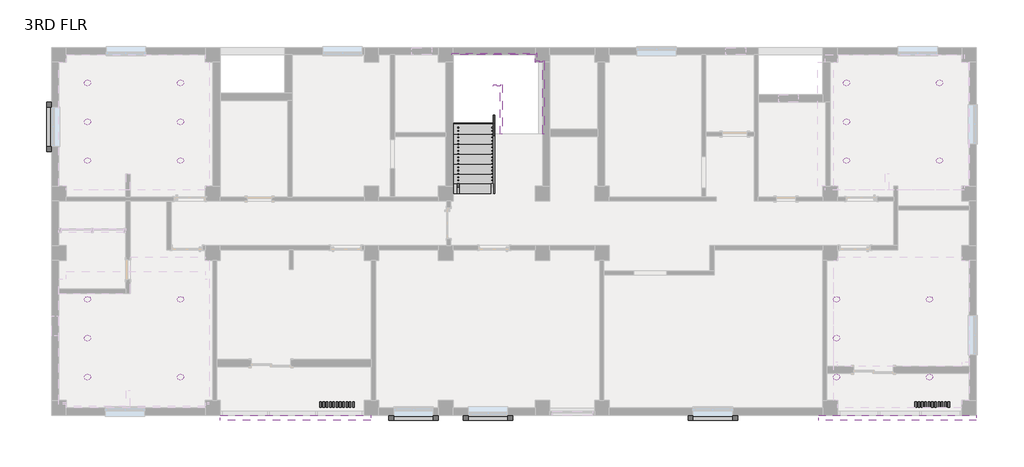
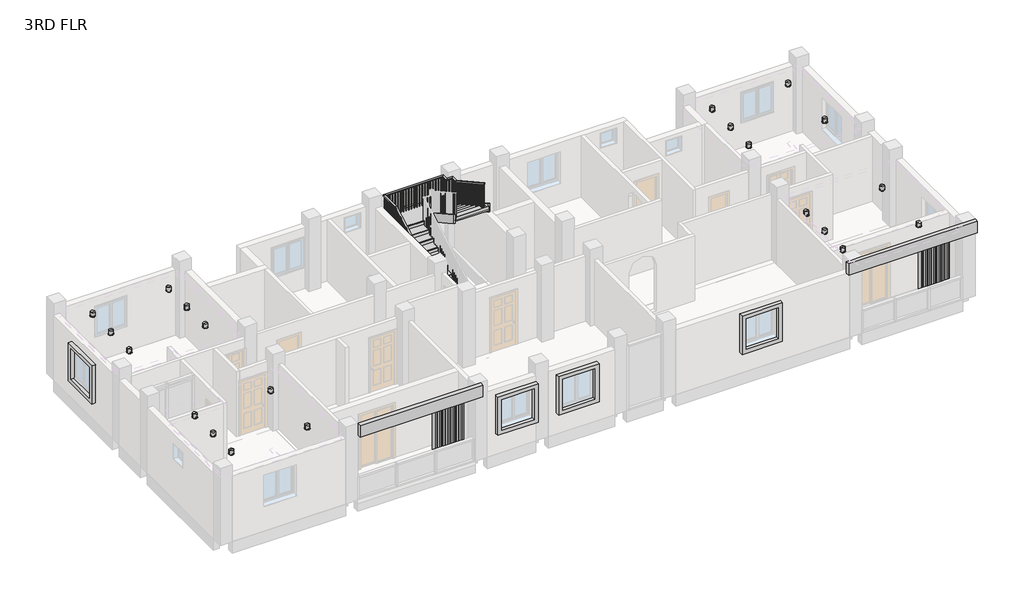
# One storey, part 5 of 5: 21 light fixtures, 8 members, 8 proxies, 1 railing, 1 stair flight.
"""IFC4 building model written with IfcOpenShell, lengths in millimetres."""

from ifc_helpers import new_model, si_unit, frame, origin, place, context, project, spatial, polyline, outline, extrude, faceted_brep, transform, mapped, element, save
from components import generic_models_11_generic_models_4_fdae65e2, generic_models_12_generic_models_6_f1297f64, generic_models_17_generic_models_17_4194431e, generic_models_21_generic_models_21_07dc1754, generic_models_4_generic_models_4_029e57d7, light_modern_pendant_14774_baffle_cc9af11b, light_modern_pendant_14774_baffle_b3430626, stair_flight_75ba705f

model = new_model("IFC4")

# Units and contexts
model_context = context("Model", 3, world=origin())
ifc_project = project(units=[si_unit("LENGTHUNIT", "METRE", prefix="MILLI")], contexts=[model_context])

# Site, building, storey
site = spatial("IfcSite", under=ifc_project)
building = spatial("IfcBuilding", under=site)
storey = spatial("IfcBuildingStorey", under=building, Name="3RD FLR", Elevation=9448.8)

# Proxies
placement = place(None, origin())
generic_models_11_generic_models_4_shape = generic_models_11_generic_models_4_fdae65e2(model_context)
element("IfcBuildingElementProxy", 1, Name="Generic Models 11 : Generic Models 4", ObjectType="Generic Models 11 : Generic Models 4", at=placement, inside=storey, context=model_context, shape_type="MappedRepresentation", body=[
    mapped(generic_models_11_generic_models_4_shape, transform((18611.1584144, 0.0, 0.0), x_axis=(1.0, 0.0, 0.0), y_axis=(0.0, 1.0, 0.0), z_axis=(0.0, 0.0, 1.0))),
])
generic_models_12_generic_models_6_shape = generic_models_12_generic_models_6_f1297f64(model_context)
element("IfcBuildingElementProxy", 2, Name="Generic Models 12 : Generic Models 6", ObjectType="Generic Models 12 : Generic Models 6", at=placement, inside=storey, context=model_context, shape_type="MappedRepresentation", body=[
    mapped(generic_models_12_generic_models_6_shape, transform((18288.0, 228.6, 0.0), x_axis=(1.0, 0.0, 0.0), y_axis=(0.0, 1.0, 0.0), z_axis=(0.0, 0.0, 1.0))),
])
generic_models_17_generic_models_17_shape = generic_models_17_generic_models_17_4194431e(model_context)
element("IfcBuildingElementProxy", 3, Name="Generic Models 17 : Generic Models 17", ObjectType="Generic Models 17 : Generic Models 17", at=placement, inside=storey, context=model_context, shape_type="MappedRepresentation", body=[
    mapped(generic_models_17_generic_models_17_shape, transform((0.0, 0.0, 0.0), x_axis=(1.0, 0.0, 0.0), y_axis=(0.0, 1.0, 0.0), z_axis=(0.0, 0.0, 1.0))),
])
generic_models_21_generic_models_21_shape = generic_models_21_generic_models_21_07dc1754(model_context)
element("IfcBuildingElementProxy", 4, Name="Generic Models 21 : Generic Models 21", ObjectType="Generic Models 21 : Generic Models 21", at=placement, inside=storey, context=model_context, shape_type="MappedRepresentation", body=[
    mapped(generic_models_21_generic_models_21_shape, transform((0.0, 0.0, 0.0), x_axis=(1.0, 0.0, 0.0), y_axis=(0.0, 1.0, 0.0), z_axis=(0.0, 0.0, 1.0))),
])
element("IfcBuildingElementProxy", 5, Name="Generic Models 25 : Generic Models 21", ObjectType="Generic Models 25 : Generic Models 21", at=placement, inside=storey, context=model_context, shape_type="MappedRepresentation", body=[
    mapped(generic_models_21_generic_models_21_shape, transform((-6905.3372689, 0.0, 0.0), x_axis=(1.0, 0.0, 0.0), y_axis=(0.0, 1.0, 0.0), z_axis=(0.0, 0.0, 1.0))),
])
element("IfcBuildingElementProxy", 6, Name="Generic Models 31 : Generic Models 21", ObjectType="Generic Models 31 : Generic Models 21", at=placement, inside=storey, context=model_context, shape_type="MappedRepresentation", body=[
    mapped(generic_models_21_generic_models_21_shape, transform((-9191.3372689, 0.0, 0.0), x_axis=(1.0, 0.0, 0.0), y_axis=(0.0, 1.0, 0.0), z_axis=(0.0, 0.0, 1.0))),
])
generic_models_4_generic_models_4_shape = generic_models_4_generic_models_4_029e57d7(model_context)
element("IfcBuildingElementProxy", 7, Name="Generic Models 4 : Generic Models 4", ObjectType="Generic Models 4 : Generic Models 4", at=placement, inside=storey, context=model_context, shape_type="MappedRepresentation", body=[
    mapped(generic_models_4_generic_models_4_shape, transform((0.0, 0.0, 0.0), x_axis=(1.0, 0.0, 0.0), y_axis=(0.0, 1.0, 0.0), z_axis=(0.0, 0.0, 1.0))),
])
element("IfcBuildingElementProxy", 8, Name="Generic Models 6 : Generic Models 6", ObjectType="Generic Models 6 : Generic Models 6", at=placement, inside=storey, context=model_context, shape_type="MappedRepresentation", body=[
    mapped(generic_models_12_generic_models_6_shape, transform((0.0, 228.6, 0.0), x_axis=(1.0, 0.0, 0.0), y_axis=(0.0, 1.0, 0.0), z_axis=(0.0, 0.0, 1.0))),
])

# Light fixtures
light_modern_pendant_14774_baffle_shape = light_modern_pendant_14774_baffle_cc9af11b(model_context)
element("IfcLightFixture", 9, ObjectType="LIGHT_-_MODERN_PENDANT_14774 : Baffle", at=placement, inside=storey, context=model_context, shape_type="MappedRepresentation", body=[
    mapped(light_modern_pendant_14774_baffle_shape, transform((-14269.0456086, -897.3794704, 9575.8), x_axis=(1.0, 0.0, 0.0), y_axis=(0.0, 1.0, 0.0), z_axis=(0.0, 0.0, 1.0))),
])
element("IfcLightFixture", 10, ObjectType="LIGHT_-_MODERN_PENDANT_14774 : Baffle", at=placement, inside=storey, context=model_context, shape_type="MappedRepresentation", body=[
    mapped(light_modern_pendant_14774_baffle_shape, transform((-14269.0456086, -3284.9794704, 9575.8), x_axis=(1.0, 0.0, 0.0), y_axis=(0.0, 1.0, 0.0), z_axis=(0.0, 0.0, 1.0))),
])
element("IfcLightFixture", 11, ObjectType="LIGHT_-_MODERN_PENDANT_14774 : Baffle", at=placement, inside=storey, context=model_context, shape_type="MappedRepresentation", body=[
    mapped(light_modern_pendant_14774_baffle_shape, transform((-14269.0456086, -2091.1794704, 9575.8), x_axis=(1.0, 0.0, 0.0), y_axis=(0.0, 1.0, 0.0), z_axis=(0.0, 0.0, 1.0))),
])
element("IfcLightFixture", 12, ObjectType="LIGHT_-_MODERN_PENDANT_14774 : Baffle", at=placement, inside=storey, context=model_context, shape_type="MappedRepresentation", body=[
    mapped(light_modern_pendant_14774_baffle_shape, transform((9048.1543914, -897.3794704, 9575.8), x_axis=(1.0, 0.0, 0.0), y_axis=(0.0, 1.0, 0.0), z_axis=(0.0, 0.0, 1.0))),
])
element("IfcLightFixture", 13, ObjectType="LIGHT_-_MODERN_PENDANT_14774 : Baffle", at=placement, inside=storey, context=model_context, shape_type="MappedRepresentation", body=[
    mapped(light_modern_pendant_14774_baffle_shape, transform((9048.1543914, -3284.9794704, 9575.8), x_axis=(1.0, 0.0, 0.0), y_axis=(0.0, 1.0, 0.0), z_axis=(0.0, 0.0, 1.0))),
])
element("IfcLightFixture", 14, ObjectType="LIGHT_-_MODERN_PENDANT_14774 : Baffle", at=placement, inside=storey, context=model_context, shape_type="MappedRepresentation", body=[
    mapped(light_modern_pendant_14774_baffle_shape, transform((9048.1543914, -2091.1794704, 9575.8), x_axis=(1.0, 0.0, 0.0), y_axis=(0.0, 1.0, 0.0), z_axis=(0.0, 0.0, 1.0))),
])
element("IfcLightFixture", 15, ObjectType="LIGHT_-_MODERN_PENDANT_14774 : Baffle", at=placement, inside=storey, context=model_context, shape_type="MappedRepresentation", body=[
    mapped(light_modern_pendant_14774_baffle_shape, transform((-14269.0456086, -7552.1794704, 9575.8), x_axis=(1.0, 0.0, 0.0), y_axis=(0.0, 1.0, 0.0), z_axis=(0.0, 0.0, 1.0))),
])
element("IfcLightFixture", 16, ObjectType="LIGHT_-_MODERN_PENDANT_14774 : Baffle", at=placement, inside=storey, context=model_context, shape_type="MappedRepresentation", body=[
    mapped(light_modern_pendant_14774_baffle_shape, transform((-14269.0456086, -9939.7794704, 9575.8), x_axis=(1.0, 0.0, 0.0), y_axis=(0.0, 1.0, 0.0), z_axis=(0.0, 0.0, 1.0))),
])
element("IfcLightFixture", 17, ObjectType="LIGHT_-_MODERN_PENDANT_14774 : Baffle", at=placement, inside=storey, context=model_context, shape_type="MappedRepresentation", body=[
    mapped(light_modern_pendant_14774_baffle_shape, transform((-14269.0456086, -8745.9794704, 9575.8), x_axis=(1.0, 0.0, 0.0), y_axis=(0.0, 1.0, 0.0), z_axis=(0.0, 0.0, 1.0))),
])
element("IfcLightFixture", 18, ObjectType="LIGHT_-_MODERN_PENDANT_14774 : Baffle", at=placement, inside=storey, context=model_context, shape_type="MappedRepresentation", body=[
    mapped(light_modern_pendant_14774_baffle_shape, transform((8743.3543914, -7552.1794704, 9575.8), x_axis=(1.0, 0.0, 0.0), y_axis=(0.0, 1.0, 0.0), z_axis=(0.0, 0.0, 1.0))),
])
element("IfcLightFixture", 19, ObjectType="LIGHT_-_MODERN_PENDANT_14774 : Baffle", at=placement, inside=storey, context=model_context, shape_type="MappedRepresentation", body=[
    mapped(light_modern_pendant_14774_baffle_shape, transform((8743.3543914, -9939.7794704, 9575.8), x_axis=(1.0, 0.0, 0.0), y_axis=(0.0, 1.0, 0.0), z_axis=(0.0, 0.0, 1.0))),
])
element("IfcLightFixture", 20, ObjectType="LIGHT_-_MODERN_PENDANT_14774 : Baffle", at=placement, inside=storey, context=model_context, shape_type="MappedRepresentation", body=[
    mapped(light_modern_pendant_14774_baffle_shape, transform((8743.3543914, -8745.9794704, 9575.8), x_axis=(1.0, 0.0, 0.0), y_axis=(0.0, 1.0, 0.0), z_axis=(0.0, 0.0, 1.0))),
])
light_modern_pendant_14774_baffle_2_shape = light_modern_pendant_14774_baffle_b3430626(model_context)
element("IfcLightFixture", 21, ObjectType="LIGHT_-_MODERN_PENDANT_14774 : Baffle", at=placement, inside=storey, context=model_context, shape_type="MappedRepresentation", body=[
    mapped(light_modern_pendant_14774_baffle_2_shape, transform((-11411.5456086, -897.3794704, 9575.8), x_axis=(-1.0, 0.0, 0.0), y_axis=(0.0, -1.0, 0.0), z_axis=(0.0, 0.0, 1.0))),
])
element("IfcLightFixture", 22, ObjectType="LIGHT_-_MODERN_PENDANT_14774 : Baffle", at=placement, inside=storey, context=model_context, shape_type="MappedRepresentation", body=[
    mapped(light_modern_pendant_14774_baffle_2_shape, transform((-11411.5456086, -3284.9794704, 9575.8), x_axis=(-1.0, 0.0, 0.0), y_axis=(0.0, -1.0, 0.0), z_axis=(0.0, 0.0, 1.0))),
])
element("IfcLightFixture", 23, ObjectType="LIGHT_-_MODERN_PENDANT_14774 : Baffle", at=placement, inside=storey, context=model_context, shape_type="MappedRepresentation", body=[
    mapped(light_modern_pendant_14774_baffle_2_shape, transform((-11411.5456086, -2091.1794704, 9575.8), x_axis=(-1.0, 0.0, 0.0), y_axis=(0.0, -1.0, 0.0), z_axis=(0.0, 0.0, 1.0))),
])
element("IfcLightFixture", 24, ObjectType="LIGHT_-_MODERN_PENDANT_14774 : Baffle", at=placement, inside=storey, context=model_context, shape_type="MappedRepresentation", body=[
    mapped(light_modern_pendant_14774_baffle_2_shape, transform((11905.6543914, -897.3794704, 9575.8), x_axis=(-1.0, 0.0, 0.0), y_axis=(0.0, -1.0, 0.0), z_axis=(0.0, 0.0, 1.0))),
])
element("IfcLightFixture", 25, ObjectType="LIGHT_-_MODERN_PENDANT_14774 : Baffle", at=placement, inside=storey, context=model_context, shape_type="MappedRepresentation", body=[
    mapped(light_modern_pendant_14774_baffle_2_shape, transform((11905.6543914, -3284.9794704, 9575.8), x_axis=(-1.0, 0.0, 0.0), y_axis=(0.0, -1.0, 0.0), z_axis=(0.0, 0.0, 1.0))),
])
element("IfcLightFixture", 26, ObjectType="LIGHT_-_MODERN_PENDANT_14774 : Baffle", at=placement, inside=storey, context=model_context, shape_type="MappedRepresentation", body=[
    mapped(light_modern_pendant_14774_baffle_2_shape, transform((-11411.5456086, -7552.1794704, 9575.8), x_axis=(-1.0, 0.0, 0.0), y_axis=(0.0, -1.0, 0.0), z_axis=(0.0, 0.0, 1.0))),
])
element("IfcLightFixture", 27, ObjectType="LIGHT_-_MODERN_PENDANT_14774 : Baffle", at=placement, inside=storey, context=model_context, shape_type="MappedRepresentation", body=[
    mapped(light_modern_pendant_14774_baffle_2_shape, transform((-11411.5456086, -9939.7794704, 9575.8), x_axis=(-1.0, 0.0, 0.0), y_axis=(0.0, -1.0, 0.0), z_axis=(0.0, 0.0, 1.0))),
])
element("IfcLightFixture", 28, ObjectType="LIGHT_-_MODERN_PENDANT_14774 : Baffle", at=placement, inside=storey, context=model_context, shape_type="MappedRepresentation", body=[
    mapped(light_modern_pendant_14774_baffle_2_shape, transform((11600.8543914, -7552.1794704, 9575.8), x_axis=(-1.0, 0.0, 0.0), y_axis=(0.0, -1.0, 0.0), z_axis=(0.0, 0.0, 1.0))),
])
element("IfcLightFixture", 29, ObjectType="LIGHT_-_MODERN_PENDANT_14774 : Baffle", at=placement, inside=storey, context=model_context, shape_type="MappedRepresentation", body=[
    mapped(light_modern_pendant_14774_baffle_2_shape, transform((11600.8543914, -9939.7794704, 9575.8), x_axis=(-1.0, 0.0, 0.0), y_axis=(0.0, -1.0, 0.0), z_axis=(0.0, 0.0, 1.0))),
])

# Members
element("IfcMember", 30, ObjectType="Stringer - 2\" Width", at=placement, inside=storey, context=model_context, shape_type="SweptSolid", body=[
    extrude(outline(polyline([(-4300.9794704, 9448.8), (-4300.9794704, 9656.3983948), (-879.896581, 11557.0), (-252.2749676, 11557.0), (-4047.0349676, 9448.8), (-4300.9794704, 9448.8)])), frame((-3080.3456086, 0.0, 0.0), z_axis=(1.0, 0.0, 0.0), x_axis=(0.0, 1.0, 0.0)), (0.0, 0.0, 1.0), 50.8),
])
element("IfcMember", 31, ObjectType="Stringer - 2\" Width", at=placement, inside=storey, context=model_context, shape_type="SweptSolid", body=[
    extrude(outline(polyline([(-3080.3456086, -33.7794704), (-3080.3456086, 17.0205296), (-467.6083398, 17.0205296), (-518.4083398, -33.7794704), (-3080.3456086, -33.7794704)])), frame((0.0, 0.0, 11252.2), z_axis=(0.0, 0.0, 1.0), x_axis=(1.0, 0.0, 0.0)), (0.0, 0.0, 1.0), 304.8),
])
element("IfcMember", 32, ObjectType="Stringer - 2\" Width", at=placement, inside=storey, context=model_context, shape_type="SweptSolid", body=[
    extrude(outline(polyline([(-518.4083398, -33.7794704), (-467.6083398, 17.0205296), (-467.6083398, -211.5794704), (-518.4083398, -262.3794704), (-518.4083398, -33.7794704)])), frame((0.0, 0.0, 11252.2), z_axis=(0.0, 0.0, 1.0), x_axis=(1.0, 0.0, 0.0)), (0.0, 0.0, 1.0), 304.8),
])
element("IfcMember", 33, ObjectType="Stringer - 2\" Width", at=placement, inside=storey, context=model_context, shape_type="SweptSolid", body=[
    extrude(outline(polyline([(-518.4083398, -262.3794704), (-467.6083398, -211.5794704), (-289.8083398, -211.5794704), (-289.8083398, -262.3794704), (-518.4083398, -262.3794704)])), frame((0.0, 0.0, 11252.2), z_axis=(0.0, 0.0, 1.0), x_axis=(1.0, 0.0, 0.0)), (0.0, 0.0, 1.0), 304.8),
])
element("IfcMember", 34, ObjectType="Stringer - 2\" Width", at=placement, inside=storey, context=model_context, shape_type="SweptSolid", body=[
    extrude(outline(polyline([(-211.5794704, 11279.1761726), (-211.5794704, 11252.2), (-790.6439732, 11252.2), (-2472.1794704, 12186.3863873), (-2472.1794704, 12535.0650614), (-211.5794704, 11279.1761726)])), frame((-289.8083398, 0.0, 0.0), z_axis=(1.0, 0.0, 0.0), x_axis=(0.0, 1.0, 0.0)), (0.0, 0.0, 1.0), 50.8),
])
element("IfcMember", 35, ObjectType="Stringer - 2\" Width", at=placement, inside=storey, context=model_context, shape_type="SweptSolid", body=[
    extrude(outline(polyline([(-4300.9794704, 9448.8), (-4300.9794704, 9656.3983948), (-998.9794704, 11490.8428392), (-998.9794704, 11142.1641651), (-4047.0349676, 9448.8), (-4300.9794704, 9448.8)])), frame((-1810.3456086, 0.0, 0.0), z_axis=(1.0, 0.0, 0.0), x_axis=(0.0, 1.0, 0.0)), (0.0, 0.0, 1.0), 50.8),
])
element("IfcMember", 36, ObjectType="Stringer - 2\" Width", at=placement, inside=storey, context=model_context, shape_type="SweptSolid", body=[
    extrude(outline(polyline([(-1810.3456086, -998.9794704), (-1810.3456086, -948.1794704), (-1585.2083398, -948.1794704), (-1585.2083398, -998.9794704), (-1810.3456086, -998.9794704)])), frame((0.0, 0.0, 11252.2), z_axis=(0.0, 0.0, 1.0), x_axis=(1.0, 0.0, 0.0)), (0.0, 0.0, 1.0), 304.8),
])
element("IfcMember", 37, ObjectType="Stringer - 2\" Width", at=placement, inside=storey, context=model_context, shape_type="SweptSolid", body=[
    extrude(outline(polyline([(-948.1794704, 11688.3983948), (-948.1794704, 11339.7197207), (-2472.1794704, 12186.3863873), (-2472.1794704, 12535.0650614), (-948.1794704, 11688.3983948)])), frame((-1585.2083398, 0.0, 0.0), z_axis=(1.0, 0.0, 0.0), x_axis=(0.0, 1.0, 0.0)), (0.0, 0.0, 1.0), 50.8),
])

# Railing
element("IfcRailing", 38, ObjectType="Handrail - Rectangular", at=placement, inside=storey, context=model_context, shape_type="SolidModel", body=[
    faceted_brep([(-2902.5456086, -4300.9794704, 10532.5333333), (-2902.5456086, -4300.9794704, 10474.420221), (-2851.7456086, -4300.9794704, 10474.420221), (-2851.7456086, -4300.9794704, 10532.5333333), (-2902.5456086, -948.1794704, 12395.2), (-2902.5456086, -935.0158682, 12344.4), (-2851.7456086, -935.0158682, 12344.4), (-2851.7456086, -948.1794704, 12395.2), (-2902.5456086, -160.7794704, 12395.2), (-2902.5456086, -160.7794704, 12344.4), (-2851.7456086, -211.5794704, 12344.4), (-2851.7456086, -211.5794704, 12395.2), (-645.4083398, -160.7794704, 12395.2), (-645.4083398, -160.7794704, 12344.4), (-696.2083398, -211.5794704, 12344.4), (-696.2083398, -211.5794704, 12395.2), (-645.4083398, -389.3794704, 12395.2), (-645.4083398, -389.3794704, 12344.4), (-696.2083398, -440.1794704, 12344.4), (-696.2083398, -440.1794704, 12395.2), (-416.8083398, -389.3794704, 12395.2), (-416.8083398, -389.3794704, 12344.4), (-467.6083398, -440.1794704, 12344.4), (-467.6083398, -440.1794704, 12395.2), (-416.8083398, -643.3794704, 12395.2), (-416.8083398, -656.5430727, 12344.4), (-467.6083398, -656.5430727, 12344.4), (-467.6083398, -643.3794704, 12395.2), (-416.8083398, -2472.1794704, 13411.2), (-467.6083398, -2472.1794704, 13411.2), (-467.6083398, -2472.1794704, 13353.0868876), (-416.8083398, -2472.1794704, 13353.0868876)], [[[0, 1, 2, 3]], [[1, 0, 4, 5]], [[2, 1, 5, 6]], [[3, 2, 6, 7]], [[0, 3, 7, 4]], [[5, 4, 8, 9]], [[6, 5, 9, 10]], [[7, 6, 10, 11]], [[4, 7, 11, 8]], [[9, 8, 12, 13]], [[10, 9, 13, 14]], [[11, 10, 14, 15]], [[8, 11, 15, 12]], [[13, 12, 16, 17]], [[14, 13, 17, 18]], [[15, 14, 18, 19]], [[12, 15, 19, 16]], [[17, 16, 20, 21]], [[18, 17, 21, 22]], [[19, 18, 22, 23]], [[16, 19, 23, 20]], [[21, 20, 24, 25]], [[22, 21, 25, 26]], [[23, 22, 26, 27]], [[20, 23, 27, 24]], [[28, 29, 30, 31]], [[25, 24, 28, 31]], [[26, 25, 31, 30]], [[27, 26, 30, 29]], [[24, 27, 29, 28]]]),
    extrude(outline(polyline([(-2437.2544704, 13333.6841099), (-2437.2544704, 12327.4666667), (-2456.3044704, 12327.4666667), (-2456.3044704, 13344.2674432), (-2437.2544704, 13333.6841099)])), frame((-451.7333398, 0.0, 0.0), z_axis=(1.0, 0.0, 0.0), x_axis=(0.0, 1.0, 0.0)), (0.0, 0.0, 1.0), 19.05),
    extrude(outline(polyline([(-2335.6544704, 13277.2396654), (-2335.6544704, 12327.4666667), (-2354.7044704, 12327.4666667), (-2354.7044704, 13287.8229988), (-2335.6544704, 13277.2396654)])), frame((-451.7333398, 0.0, 0.0), z_axis=(1.0, 0.0, 0.0), x_axis=(0.0, 1.0, 0.0)), (0.0, 0.0, 1.0), 19.05),
    extrude(outline(polyline([(-2234.0544704, 13220.795221), (-2234.0544704, 12327.4666667), (-2253.1044704, 12327.4666667), (-2253.1044704, 13231.3785543), (-2234.0544704, 13220.795221)])), frame((-451.7333398, 0.0, 0.0), z_axis=(1.0, 0.0, 0.0), x_axis=(0.0, 1.0, 0.0)), (0.0, 0.0, 1.0), 19.05),
    extrude(outline(polyline([(-2132.4544704, 13164.3507765), (-2132.4544704, 12158.1333333), (-2151.5044704, 12158.1333333), (-2151.5044704, 13174.9341099), (-2132.4544704, 13164.3507765)])), frame((-451.7333398, 0.0, 0.0), z_axis=(1.0, 0.0, 0.0), x_axis=(0.0, 1.0, 0.0)), (0.0, 0.0, 1.0), 19.05),
    extrude(outline(polyline([(-2030.8544704, 13107.9063321), (-2030.8544704, 12158.1333333), (-2049.9044704, 12158.1333333), (-2049.9044704, 13118.4896654), (-2030.8544704, 13107.9063321)])), frame((-451.7333398, 0.0, 0.0), z_axis=(1.0, 0.0, 0.0), x_axis=(0.0, 1.0, 0.0)), (0.0, 0.0, 1.0), 19.05),
    extrude(outline(polyline([(-1929.2544704, 13051.4618876), (-1929.2544704, 12158.1333333), (-1948.3044704, 12158.1333333), (-1948.3044704, 13062.045221), (-1929.2544704, 13051.4618876)])), frame((-451.7333398, 0.0, 0.0), z_axis=(1.0, 0.0, 0.0), x_axis=(0.0, 1.0, 0.0)), (0.0, 0.0, 1.0), 19.05),
    extrude(outline(polyline([(-1827.6544704, 12995.0174432), (-1827.6544704, 11988.8), (-1846.7044704, 11988.8), (-1846.7044704, 13005.6007765), (-1827.6544704, 12995.0174432)])), frame((-451.7333398, 0.0, 0.0), z_axis=(1.0, 0.0, 0.0), x_axis=(0.0, 1.0, 0.0)), (0.0, 0.0, 1.0), 19.05),
    extrude(outline(polyline([(-1726.0544704, 12938.5729988), (-1726.0544704, 11988.8), (-1745.1044704, 11988.8), (-1745.1044704, 12949.1563321), (-1726.0544704, 12938.5729988)])), frame((-451.7333398, 0.0, 0.0), z_axis=(1.0, 0.0, 0.0), x_axis=(0.0, 1.0, 0.0)), (0.0, 0.0, 1.0), 19.05),
    extrude(outline(polyline([(-1624.4544704, 12882.1285543), (-1624.4544704, 11988.8), (-1643.5044704, 11988.8), (-1643.5044704, 12892.7118876), (-1624.4544704, 12882.1285543)])), frame((-451.7333398, 0.0, 0.0), z_axis=(1.0, 0.0, 0.0), x_axis=(0.0, 1.0, 0.0)), (0.0, 0.0, 1.0), 19.05),
    extrude(outline(polyline([(-1522.8544704, 12825.6841099), (-1522.8544704, 11819.4666667), (-1541.9044704, 11819.4666667), (-1541.9044704, 12836.2674432), (-1522.8544704, 12825.6841099)])), frame((-451.7333398, 0.0, 0.0), z_axis=(1.0, 0.0, 0.0), x_axis=(0.0, 1.0, 0.0)), (0.0, 0.0, 1.0), 19.05),
    extrude(outline(polyline([(-1421.2544704, 12769.2396654), (-1421.2544704, 11819.4666667), (-1440.3044704, 11819.4666667), (-1440.3044704, 12779.8229988), (-1421.2544704, 12769.2396654)])), frame((-451.7333398, 0.0, 0.0), z_axis=(1.0, 0.0, 0.0), x_axis=(0.0, 1.0, 0.0)), (0.0, 0.0, 1.0), 19.05),
    extrude(outline(polyline([(-1319.6544704, 12712.795221), (-1319.6544704, 11819.4666667), (-1338.7044704, 11819.4666667), (-1338.7044704, 12723.3785543), (-1319.6544704, 12712.795221)])), frame((-451.7333398, 0.0, 0.0), z_axis=(1.0, 0.0, 0.0), x_axis=(0.0, 1.0, 0.0)), (0.0, 0.0, 1.0), 19.05),
    extrude(outline(polyline([(-1218.0544704, 12656.3507765), (-1218.0544704, 11650.1333333), (-1237.1044704, 11650.1333333), (-1237.1044704, 12666.9341099), (-1218.0544704, 12656.3507765)])), frame((-451.7333398, 0.0, 0.0), z_axis=(1.0, 0.0, 0.0), x_axis=(0.0, 1.0, 0.0)), (0.0, 0.0, 1.0), 19.05),
    extrude(outline(polyline([(-1116.4544704, 12599.9063321), (-1116.4544704, 11650.1333333), (-1135.5044704, 11650.1333333), (-1135.5044704, 12610.4896654), (-1116.4544704, 12599.9063321)])), frame((-451.7333398, 0.0, 0.0), z_axis=(1.0, 0.0, 0.0), x_axis=(0.0, 1.0, 0.0)), (0.0, 0.0, 1.0), 19.05),
    extrude(outline(polyline([(-1014.8544704, 12543.4618876), (-1014.8544704, 11650.1333333), (-1033.9044704, 11650.1333333), (-1033.9044704, 12554.045221), (-1014.8544704, 12543.4618876)])), frame((-451.7333398, 0.0, 0.0), z_axis=(1.0, 0.0, 0.0), x_axis=(0.0, 1.0, 0.0)), (0.0, 0.0, 1.0), 19.05),
    extrude(outline(polyline([(-913.2544704, 12487.0174432), (-913.2544704, 11480.8), (-932.3044704, 11480.8), (-932.3044704, 12497.6007765), (-913.2544704, 12487.0174432)])), frame((-451.7333398, 0.0, 0.0), z_axis=(1.0, 0.0, 0.0), x_axis=(0.0, 1.0, 0.0)), (0.0, 0.0, 1.0), 19.05),
    extrude(outline(polyline([(-811.6544704, 12430.5729988), (-811.6544704, 11480.8), (-830.7044704, 11480.8), (-830.7044704, 12441.1563321), (-811.6544704, 12430.5729988)])), frame((-451.7333398, 0.0, 0.0), z_axis=(1.0, 0.0, 0.0), x_axis=(0.0, 1.0, 0.0)), (0.0, 0.0, 1.0), 19.05),
    extrude(outline(polyline([(-710.0544704, 12374.1285543), (-710.0544704, 11480.8), (-729.1044704, 11480.8), (-729.1044704, 12384.7118876), (-710.0544704, 12374.1285543)])), frame((-451.7333398, 0.0, 0.0), z_axis=(1.0, 0.0, 0.0), x_axis=(0.0, 1.0, 0.0)), (0.0, 0.0, 1.0), 19.05),
    extrude(outline(polyline([(-432.6833398, -608.4544704), (-432.6833398, -627.5044704), (-451.7333398, -627.5044704), (-451.7333398, -608.4544704), (-432.6833398, -608.4544704)])), frame((0.0, 0.0, 11480.8), z_axis=(0.0, 0.0, 1.0), x_axis=(1.0, 0.0, 0.0)), (0.0, 0.0, 1.0), 863.6),
    extrude(outline(polyline([(-432.6833398, -506.8544704), (-432.6833398, -525.9044704), (-451.7333398, -525.9044704), (-451.7333398, -506.8544704), (-432.6833398, -506.8544704)])), frame((0.0, 0.0, 11480.8), z_axis=(0.0, 0.0, 1.0), x_axis=(1.0, 0.0, 0.0)), (0.0, 0.0, 1.0), 863.6),
    extrude(outline(polyline([(-477.1333398, -405.2544704), (-458.0833398, -405.2544704), (-458.0833398, -424.3044704), (-477.1333398, -424.3044704), (-477.1333398, -405.2544704)])), frame((0.0, 0.0, 11480.8), z_axis=(0.0, 0.0, 1.0), x_axis=(1.0, 0.0, 0.0)), (0.0, 0.0, 1.0), 863.6),
    extrude(outline(polyline([(-578.7333398, -405.2544704), (-559.6833398, -405.2544704), (-559.6833398, -424.3044704), (-578.7333398, -424.3044704), (-578.7333398, -405.2544704)])), frame((0.0, 0.0, 11480.8), z_axis=(0.0, 0.0, 1.0), x_axis=(1.0, 0.0, 0.0)), (0.0, 0.0, 1.0), 863.6),
    extrude(outline(polyline([(-661.2833398, -379.8544704), (-661.2833398, -398.9044704), (-680.3333398, -398.9044704), (-680.3333398, -379.8544704), (-661.2833398, -379.8544704)])), frame((0.0, 0.0, 11480.8), z_axis=(0.0, 0.0, 1.0), x_axis=(1.0, 0.0, 0.0)), (0.0, 0.0, 1.0), 863.6),
    extrude(outline(polyline([(-661.2833398, -278.2544704), (-661.2833398, -297.3044704), (-680.3333398, -297.3044704), (-680.3333398, -278.2544704), (-661.2833398, -278.2544704)])), frame((0.0, 0.0, 11480.8), z_axis=(0.0, 0.0, 1.0), x_axis=(1.0, 0.0, 0.0)), (0.0, 0.0, 1.0), 863.6),
    extrude(outline(polyline([(-753.0706086, -176.6544704), (-734.0206086, -176.6544704), (-734.0206086, -195.7044704), (-753.0706086, -195.7044704), (-753.0706086, -176.6544704)])), frame((0.0, 0.0, 11480.8), z_axis=(0.0, 0.0, 1.0), x_axis=(1.0, 0.0, 0.0)), (0.0, 0.0, 1.0), 863.6),
    extrude(outline(polyline([(-854.6706086, -176.6544704), (-835.6206086, -176.6544704), (-835.6206086, -195.7044704), (-854.6706086, -195.7044704), (-854.6706086, -176.6544704)])), frame((0.0, 0.0, 11480.8), z_axis=(0.0, 0.0, 1.0), x_axis=(1.0, 0.0, 0.0)), (0.0, 0.0, 1.0), 863.6),
    extrude(outline(polyline([(-956.2706086, -176.6544704), (-937.2206086, -176.6544704), (-937.2206086, -195.7044704), (-956.2706086, -195.7044704), (-956.2706086, -176.6544704)])), frame((0.0, 0.0, 11480.8), z_axis=(0.0, 0.0, 1.0), x_axis=(1.0, 0.0, 0.0)), (0.0, 0.0, 1.0), 863.6),
    extrude(outline(polyline([(-1057.8706086, -176.6544704), (-1038.8206086, -176.6544704), (-1038.8206086, -195.7044704), (-1057.8706086, -195.7044704), (-1057.8706086, -176.6544704)])), frame((0.0, 0.0, 11480.8), z_axis=(0.0, 0.0, 1.0), x_axis=(1.0, 0.0, 0.0)), (0.0, 0.0, 1.0), 863.6),
    extrude(outline(polyline([(-1159.4706086, -176.6544704), (-1140.4206086, -176.6544704), (-1140.4206086, -195.7044704), (-1159.4706086, -195.7044704), (-1159.4706086, -176.6544704)])), frame((0.0, 0.0, 11480.8), z_axis=(0.0, 0.0, 1.0), x_axis=(1.0, 0.0, 0.0)), (0.0, 0.0, 1.0), 863.6),
    extrude(outline(polyline([(-1261.0706086, -176.6544704), (-1242.0206086, -176.6544704), (-1242.0206086, -195.7044704), (-1261.0706086, -195.7044704), (-1261.0706086, -176.6544704)])), frame((0.0, 0.0, 11480.8), z_axis=(0.0, 0.0, 1.0), x_axis=(1.0, 0.0, 0.0)), (0.0, 0.0, 1.0), 863.6),
    extrude(outline(polyline([(-1362.6706086, -176.6544704), (-1343.6206086, -176.6544704), (-1343.6206086, -195.7044704), (-1362.6706086, -195.7044704), (-1362.6706086, -176.6544704)])), frame((0.0, 0.0, 11480.8), z_axis=(0.0, 0.0, 1.0), x_axis=(1.0, 0.0, 0.0)), (0.0, 0.0, 1.0), 863.6),
    extrude(outline(polyline([(-1464.2706086, -176.6544704), (-1445.2206086, -176.6544704), (-1445.2206086, -195.7044704), (-1464.2706086, -195.7044704), (-1464.2706086, -176.6544704)])), frame((0.0, 0.0, 11480.8), z_axis=(0.0, 0.0, 1.0), x_axis=(1.0, 0.0, 0.0)), (0.0, 0.0, 1.0), 863.6),
    extrude(outline(polyline([(-1565.8706086, -176.6544704), (-1546.8206086, -176.6544704), (-1546.8206086, -195.7044704), (-1565.8706086, -195.7044704), (-1565.8706086, -176.6544704)])), frame((0.0, 0.0, 11480.8), z_axis=(0.0, 0.0, 1.0), x_axis=(1.0, 0.0, 0.0)), (0.0, 0.0, 1.0), 863.6),
    extrude(outline(polyline([(-1667.4706086, -176.6544704), (-1648.4206086, -176.6544704), (-1648.4206086, -195.7044704), (-1667.4706086, -195.7044704), (-1667.4706086, -176.6544704)])), frame((0.0, 0.0, 11480.8), z_axis=(0.0, 0.0, 1.0), x_axis=(1.0, 0.0, 0.0)), (0.0, 0.0, 1.0), 863.6),
    extrude(outline(polyline([(-1769.0706086, -176.6544704), (-1750.0206086, -176.6544704), (-1750.0206086, -195.7044704), (-1769.0706086, -195.7044704), (-1769.0706086, -176.6544704)])), frame((0.0, 0.0, 11480.8), z_axis=(0.0, 0.0, 1.0), x_axis=(1.0, 0.0, 0.0)), (0.0, 0.0, 1.0), 863.6),
    extrude(outline(polyline([(-1870.6706086, -176.6544704), (-1851.6206086, -176.6544704), (-1851.6206086, -195.7044704), (-1870.6706086, -195.7044704), (-1870.6706086, -176.6544704)])), frame((0.0, 0.0, 11480.8), z_axis=(0.0, 0.0, 1.0), x_axis=(1.0, 0.0, 0.0)), (0.0, 0.0, 1.0), 863.6),
    extrude(outline(polyline([(-1972.2706086, -176.6544704), (-1953.2206086, -176.6544704), (-1953.2206086, -195.7044704), (-1972.2706086, -195.7044704), (-1972.2706086, -176.6544704)])), frame((0.0, 0.0, 11480.8), z_axis=(0.0, 0.0, 1.0), x_axis=(1.0, 0.0, 0.0)), (0.0, 0.0, 1.0), 863.6),
    extrude(outline(polyline([(-2073.8706086, -176.6544704), (-2054.8206086, -176.6544704), (-2054.8206086, -195.7044704), (-2073.8706086, -195.7044704), (-2073.8706086, -176.6544704)])), frame((0.0, 0.0, 11480.8), z_axis=(0.0, 0.0, 1.0), x_axis=(1.0, 0.0, 0.0)), (0.0, 0.0, 1.0), 863.6),
    extrude(outline(polyline([(-2175.4706086, -176.6544704), (-2156.4206086, -176.6544704), (-2156.4206086, -195.7044704), (-2175.4706086, -195.7044704), (-2175.4706086, -176.6544704)])), frame((0.0, 0.0, 11480.8), z_axis=(0.0, 0.0, 1.0), x_axis=(1.0, 0.0, 0.0)), (0.0, 0.0, 1.0), 863.6),
    extrude(outline(polyline([(-2277.0706086, -176.6544704), (-2258.0206086, -176.6544704), (-2258.0206086, -195.7044704), (-2277.0706086, -195.7044704), (-2277.0706086, -176.6544704)])), frame((0.0, 0.0, 11480.8), z_axis=(0.0, 0.0, 1.0), x_axis=(1.0, 0.0, 0.0)), (0.0, 0.0, 1.0), 863.6),
    extrude(outline(polyline([(-2378.6706086, -176.6544704), (-2359.6206086, -176.6544704), (-2359.6206086, -195.7044704), (-2378.6706086, -195.7044704), (-2378.6706086, -176.6544704)])), frame((0.0, 0.0, 11480.8), z_axis=(0.0, 0.0, 1.0), x_axis=(1.0, 0.0, 0.0)), (0.0, 0.0, 1.0), 863.6),
    extrude(outline(polyline([(-2480.2706086, -176.6544704), (-2461.2206086, -176.6544704), (-2461.2206086, -195.7044704), (-2480.2706086, -195.7044704), (-2480.2706086, -176.6544704)])), frame((0.0, 0.0, 11480.8), z_axis=(0.0, 0.0, 1.0), x_axis=(1.0, 0.0, 0.0)), (0.0, 0.0, 1.0), 863.6),
    extrude(outline(polyline([(-2581.8706086, -176.6544704), (-2562.8206086, -176.6544704), (-2562.8206086, -195.7044704), (-2581.8706086, -195.7044704), (-2581.8706086, -176.6544704)])), frame((0.0, 0.0, 11480.8), z_axis=(0.0, 0.0, 1.0), x_axis=(1.0, 0.0, 0.0)), (0.0, 0.0, 1.0), 863.6),
    extrude(outline(polyline([(-2683.4706086, -176.6544704), (-2664.4206086, -176.6544704), (-2664.4206086, -195.7044704), (-2683.4706086, -195.7044704), (-2683.4706086, -176.6544704)])), frame((0.0, 0.0, 11480.8), z_axis=(0.0, 0.0, 1.0), x_axis=(1.0, 0.0, 0.0)), (0.0, 0.0, 1.0), 863.6),
    extrude(outline(polyline([(-2785.0706086, -176.6544704), (-2766.0206086, -176.6544704), (-2766.0206086, -195.7044704), (-2785.0706086, -195.7044704), (-2785.0706086, -176.6544704)])), frame((0.0, 0.0, 11480.8), z_axis=(0.0, 0.0, 1.0), x_axis=(1.0, 0.0, 0.0)), (0.0, 0.0, 1.0), 863.6),
    extrude(outline(polyline([(-2886.6706086, -246.5044704), (-2886.6706086, -227.4544704), (-2867.6206086, -227.4544704), (-2867.6206086, -246.5044704), (-2886.6706086, -246.5044704)])), frame((0.0, 0.0, 11480.8), z_axis=(0.0, 0.0, 1.0), x_axis=(1.0, 0.0, 0.0)), (0.0, 0.0, 1.0), 863.6),
    extrude(outline(polyline([(-2886.6706086, -348.1044704), (-2886.6706086, -329.0544704), (-2867.6206086, -329.0544704), (-2867.6206086, -348.1044704), (-2886.6706086, -348.1044704)])), frame((0.0, 0.0, 11480.8), z_axis=(0.0, 0.0, 1.0), x_axis=(1.0, 0.0, 0.0)), (0.0, 0.0, 1.0), 863.6),
    extrude(outline(polyline([(-2886.6706086, -449.7044704), (-2886.6706086, -430.6544704), (-2867.6206086, -430.6544704), (-2867.6206086, -449.7044704), (-2886.6706086, -449.7044704)])), frame((0.0, 0.0, 11480.8), z_axis=(0.0, 0.0, 1.0), x_axis=(1.0, 0.0, 0.0)), (0.0, 0.0, 1.0), 863.6),
    extrude(outline(polyline([(-2886.6706086, -551.3044704), (-2886.6706086, -532.2544704), (-2867.6206086, -532.2544704), (-2867.6206086, -551.3044704), (-2886.6706086, -551.3044704)])), frame((0.0, 0.0, 11480.8), z_axis=(0.0, 0.0, 1.0), x_axis=(1.0, 0.0, 0.0)), (0.0, 0.0, 1.0), 863.6),
    extrude(outline(polyline([(-2886.6706086, -652.9044704), (-2886.6706086, -633.8544704), (-2867.6206086, -633.8544704), (-2867.6206086, -652.9044704), (-2886.6706086, -652.9044704)])), frame((0.0, 0.0, 11480.8), z_axis=(0.0, 0.0, 1.0), x_axis=(1.0, 0.0, 0.0)), (0.0, 0.0, 1.0), 863.6),
    extrude(outline(polyline([(-2886.6706086, -754.5044704), (-2886.6706086, -735.4544704), (-2867.6206086, -735.4544704), (-2867.6206086, -754.5044704), (-2886.6706086, -754.5044704)])), frame((0.0, 0.0, 11480.8), z_axis=(0.0, 0.0, 1.0), x_axis=(1.0, 0.0, 0.0)), (0.0, 0.0, 1.0), 863.6),
    extrude(outline(polyline([(-2886.6706086, -856.1044704), (-2886.6706086, -837.0544704), (-2867.6206086, -837.0544704), (-2867.6206086, -856.1044704), (-2886.6706086, -856.1044704)])), frame((0.0, 0.0, 11480.8), z_axis=(0.0, 0.0, 1.0), x_axis=(1.0, 0.0, 0.0)), (0.0, 0.0, 1.0), 863.6),
    extrude(outline(polyline([(-938.6544704, 12342.3785543), (-938.6544704, 11480.8), (-957.7044704, 11480.8), (-957.7044704, 12331.795221), (-938.6544704, 12342.3785543)])), frame((-2886.6706086, 0.0, 0.0), z_axis=(1.0, 0.0, 0.0), x_axis=(0.0, 1.0, 0.0)), (0.0, 0.0, 1.0), 19.05),
    extrude(outline(polyline([(-1040.2544704, 12285.9341099), (-1040.2544704, 11311.4666667), (-1059.3044704, 11311.4666667), (-1059.3044704, 12275.3507765), (-1040.2544704, 12285.9341099)])), frame((-2886.6706086, 0.0, 0.0), z_axis=(1.0, 0.0, 0.0), x_axis=(0.0, 1.0, 0.0)), (0.0, 0.0, 1.0), 19.05),
    extrude(outline(polyline([(-1141.8544704, 12229.4896654), (-1141.8544704, 11311.4666667), (-1160.9044704, 11311.4666667), (-1160.9044704, 12218.9063321), (-1141.8544704, 12229.4896654)])), frame((-2886.6706086, 0.0, 0.0), z_axis=(1.0, 0.0, 0.0), x_axis=(0.0, 1.0, 0.0)), (0.0, 0.0, 1.0), 19.05),
    extrude(outline(polyline([(-1243.4544704, 12173.045221), (-1243.4544704, 11311.4666667), (-1262.5044704, 11311.4666667), (-1262.5044704, 12162.4618876), (-1243.4544704, 12173.045221)])), frame((-2886.6706086, 0.0, 0.0), z_axis=(1.0, 0.0, 0.0), x_axis=(0.0, 1.0, 0.0)), (0.0, 0.0, 1.0), 19.05),
    extrude(outline(polyline([(-1345.0544704, 12116.6007765), (-1345.0544704, 11142.1333333), (-1364.1044704, 11142.1333333), (-1364.1044704, 12106.0174432), (-1345.0544704, 12116.6007765)])), frame((-2886.6706086, 0.0, 0.0), z_axis=(1.0, 0.0, 0.0), x_axis=(0.0, 1.0, 0.0)), (0.0, 0.0, 1.0), 19.05),
    extrude(outline(polyline([(-1446.6544704, 12060.1563321), (-1446.6544704, 11142.1333333), (-1465.7044704, 11142.1333333), (-1465.7044704, 12049.5729988), (-1446.6544704, 12060.1563321)])), frame((-2886.6706086, 0.0, 0.0), z_axis=(1.0, 0.0, 0.0), x_axis=(0.0, 1.0, 0.0)), (0.0, 0.0, 1.0), 19.05),
    extrude(outline(polyline([(-1548.2544704, 12003.7118876), (-1548.2544704, 11142.1333333), (-1567.3044704, 11142.1333333), (-1567.3044704, 11993.1285543), (-1548.2544704, 12003.7118876)])), frame((-2886.6706086, 0.0, 0.0), z_axis=(1.0, 0.0, 0.0), x_axis=(0.0, 1.0, 0.0)), (0.0, 0.0, 1.0), 19.05),
    extrude(outline(polyline([(-1649.8544704, 11947.2674432), (-1649.8544704, 10972.8), (-1668.9044704, 10972.8), (-1668.9044704, 11936.6841099), (-1649.8544704, 11947.2674432)])), frame((-2886.6706086, 0.0, 0.0), z_axis=(1.0, 0.0, 0.0), x_axis=(0.0, 1.0, 0.0)), (0.0, 0.0, 1.0), 19.05),
    extrude(outline(polyline([(-1751.4544704, 11890.8229988), (-1751.4544704, 10972.8), (-1770.5044704, 10972.8), (-1770.5044704, 11880.2396654), (-1751.4544704, 11890.8229988)])), frame((-2886.6706086, 0.0, 0.0), z_axis=(1.0, 0.0, 0.0), x_axis=(0.0, 1.0, 0.0)), (0.0, 0.0, 1.0), 19.05),
    extrude(outline(polyline([(-1853.0544704, 11834.3785543), (-1853.0544704, 10972.8), (-1872.1044704, 10972.8), (-1872.1044704, 11823.795221), (-1853.0544704, 11834.3785543)])), frame((-2886.6706086, 0.0, 0.0), z_axis=(1.0, 0.0, 0.0), x_axis=(0.0, 1.0, 0.0)), (0.0, 0.0, 1.0), 19.05),
    extrude(outline(polyline([(-1954.6544704, 11777.9341099), (-1954.6544704, 10803.4666667), (-1973.7044704, 10803.4666667), (-1973.7044704, 11767.3507765), (-1954.6544704, 11777.9341099)])), frame((-2886.6706086, 0.0, 0.0), z_axis=(1.0, 0.0, 0.0), x_axis=(0.0, 1.0, 0.0)), (0.0, 0.0, 1.0), 19.05),
    extrude(outline(polyline([(-2056.2544704, 11721.4896654), (-2056.2544704, 10803.4666667), (-2075.3044704, 10803.4666667), (-2075.3044704, 11710.9063321), (-2056.2544704, 11721.4896654)])), frame((-2886.6706086, 0.0, 0.0), z_axis=(1.0, 0.0, 0.0), x_axis=(0.0, 1.0, 0.0)), (0.0, 0.0, 1.0), 19.05),
    extrude(outline(polyline([(-2157.8544704, 11665.045221), (-2157.8544704, 10803.4666667), (-2176.9044704, 10803.4666667), (-2176.9044704, 11654.4618876), (-2157.8544704, 11665.045221)])), frame((-2886.6706086, 0.0, 0.0), z_axis=(1.0, 0.0, 0.0), x_axis=(0.0, 1.0, 0.0)), (0.0, 0.0, 1.0), 19.05),
    extrude(outline(polyline([(-2259.4544704, 11608.6007765), (-2259.4544704, 10634.1333333), (-2278.5044704, 10634.1333333), (-2278.5044704, 11598.0174432), (-2259.4544704, 11608.6007765)])), frame((-2886.6706086, 0.0, 0.0), z_axis=(1.0, 0.0, 0.0), x_axis=(0.0, 1.0, 0.0)), (0.0, 0.0, 1.0), 19.05),
    extrude(outline(polyline([(-2361.0544704, 11552.1563321), (-2361.0544704, 10634.1333333), (-2380.1044704, 10634.1333333), (-2380.1044704, 11541.5729988), (-2361.0544704, 11552.1563321)])), frame((-2886.6706086, 0.0, 0.0), z_axis=(1.0, 0.0, 0.0), x_axis=(0.0, 1.0, 0.0)), (0.0, 0.0, 1.0), 19.05),
    extrude(outline(polyline([(-2462.6544704, 11495.7118876), (-2462.6544704, 10634.1333333), (-2481.7044704, 10634.1333333), (-2481.7044704, 11485.1285543), (-2462.6544704, 11495.7118876)])), frame((-2886.6706086, 0.0, 0.0), z_axis=(1.0, 0.0, 0.0), x_axis=(0.0, 1.0, 0.0)), (0.0, 0.0, 1.0), 19.05),
    extrude(outline(polyline([(-2564.2544704, 11439.2674432), (-2564.2544704, 10464.8), (-2583.3044704, 10464.8), (-2583.3044704, 11428.6841099), (-2564.2544704, 11439.2674432)])), frame((-2886.6706086, 0.0, 0.0), z_axis=(1.0, 0.0, 0.0), x_axis=(0.0, 1.0, 0.0)), (0.0, 0.0, 1.0), 19.05),
    extrude(outline(polyline([(-2665.8544704, 11382.8229988), (-2665.8544704, 10464.8), (-2684.9044704, 10464.8), (-2684.9044704, 11372.2396654), (-2665.8544704, 11382.8229988)])), frame((-2886.6706086, 0.0, 0.0), z_axis=(1.0, 0.0, 0.0), x_axis=(0.0, 1.0, 0.0)), (0.0, 0.0, 1.0), 19.05),
    extrude(outline(polyline([(-2767.4544704, 11326.3785543), (-2767.4544704, 10464.8), (-2786.5044704, 10464.8), (-2786.5044704, 11315.795221), (-2767.4544704, 11326.3785543)])), frame((-2886.6706086, 0.0, 0.0), z_axis=(1.0, 0.0, 0.0), x_axis=(0.0, 1.0, 0.0)), (0.0, 0.0, 1.0), 19.05),
    extrude(outline(polyline([(-2869.0544704, 11269.9341099), (-2869.0544704, 10295.4666667), (-2888.1044704, 10295.4666667), (-2888.1044704, 11259.3507765), (-2869.0544704, 11269.9341099)])), frame((-2886.6706086, 0.0, 0.0), z_axis=(1.0, 0.0, 0.0), x_axis=(0.0, 1.0, 0.0)), (0.0, 0.0, 1.0), 19.05),
    extrude(outline(polyline([(-2970.6544704, 11213.4896654), (-2970.6544704, 10295.4666667), (-2989.7044704, 10295.4666667), (-2989.7044704, 11202.9063321), (-2970.6544704, 11213.4896654)])), frame((-2886.6706086, 0.0, 0.0), z_axis=(1.0, 0.0, 0.0), x_axis=(0.0, 1.0, 0.0)), (0.0, 0.0, 1.0), 19.05),
    extrude(outline(polyline([(-3072.2544704, 11157.045221), (-3072.2544704, 10295.4666667), (-3091.3044704, 10295.4666667), (-3091.3044704, 11146.4618876), (-3072.2544704, 11157.045221)])), frame((-2886.6706086, 0.0, 0.0), z_axis=(1.0, 0.0, 0.0), x_axis=(0.0, 1.0, 0.0)), (0.0, 0.0, 1.0), 19.05),
    extrude(outline(polyline([(-3173.8544704, 11100.6007765), (-3173.8544704, 10126.1333333), (-3192.9044704, 10126.1333333), (-3192.9044704, 11090.0174432), (-3173.8544704, 11100.6007765)])), frame((-2886.6706086, 0.0, 0.0), z_axis=(1.0, 0.0, 0.0), x_axis=(0.0, 1.0, 0.0)), (0.0, 0.0, 1.0), 19.05),
    extrude(outline(polyline([(-3275.4544704, 11044.1563321), (-3275.4544704, 10126.1333333), (-3294.5044704, 10126.1333333), (-3294.5044704, 11033.5729988), (-3275.4544704, 11044.1563321)])), frame((-2886.6706086, 0.0, 0.0), z_axis=(1.0, 0.0, 0.0), x_axis=(0.0, 1.0, 0.0)), (0.0, 0.0, 1.0), 19.05),
    extrude(outline(polyline([(-3377.0544704, 10987.7118876), (-3377.0544704, 10126.1333333), (-3396.1044704, 10126.1333333), (-3396.1044704, 10977.1285543), (-3377.0544704, 10987.7118876)])), frame((-2886.6706086, 0.0, 0.0), z_axis=(1.0, 0.0, 0.0), x_axis=(0.0, 1.0, 0.0)), (0.0, 0.0, 1.0), 19.05),
    extrude(outline(polyline([(-3478.6544704, 10931.2674432), (-3478.6544704, 9956.8), (-3497.7044704, 9956.8), (-3497.7044704, 10920.6841099), (-3478.6544704, 10931.2674432)])), frame((-2886.6706086, 0.0, 0.0), z_axis=(1.0, 0.0, 0.0), x_axis=(0.0, 1.0, 0.0)), (0.0, 0.0, 1.0), 19.05),
    extrude(outline(polyline([(-3580.2544704, 10874.8229988), (-3580.2544704, 9956.8), (-3599.3044704, 9956.8), (-3599.3044704, 10864.2396654), (-3580.2544704, 10874.8229988)])), frame((-2886.6706086, 0.0, 0.0), z_axis=(1.0, 0.0, 0.0), x_axis=(0.0, 1.0, 0.0)), (0.0, 0.0, 1.0), 19.05),
    extrude(outline(polyline([(-3681.8544704, 10818.3785543), (-3681.8544704, 9956.8), (-3700.9044704, 9956.8), (-3700.9044704, 10807.795221), (-3681.8544704, 10818.3785543)])), frame((-2886.6706086, 0.0, 0.0), z_axis=(1.0, 0.0, 0.0), x_axis=(0.0, 1.0, 0.0)), (0.0, 0.0, 1.0), 19.05),
    extrude(outline(polyline([(-3783.4544704, 10761.9341099), (-3783.4544704, 9787.4666667), (-3802.5044704, 9787.4666667), (-3802.5044704, 10751.3507765), (-3783.4544704, 10761.9341099)])), frame((-2886.6706086, 0.0, 0.0), z_axis=(1.0, 0.0, 0.0), x_axis=(0.0, 1.0, 0.0)), (0.0, 0.0, 1.0), 19.05),
    extrude(outline(polyline([(-3885.0544704, 10705.4896654), (-3885.0544704, 9787.4666667), (-3904.1044704, 9787.4666667), (-3904.1044704, 10694.9063321), (-3885.0544704, 10705.4896654)])), frame((-2886.6706086, 0.0, 0.0), z_axis=(1.0, 0.0, 0.0), x_axis=(0.0, 1.0, 0.0)), (0.0, 0.0, 1.0), 19.05),
    extrude(outline(polyline([(-3986.6544704, 10649.045221), (-3986.6544704, 9787.4666667), (-4005.7044704, 9787.4666667), (-4005.7044704, 10638.4618876), (-3986.6544704, 10649.045221)])), frame((-2886.6706086, 0.0, 0.0), z_axis=(1.0, 0.0, 0.0), x_axis=(0.0, 1.0, 0.0)), (0.0, 0.0, 1.0), 19.05),
    extrude(outline(polyline([(-4088.2544704, 10592.6007765), (-4088.2544704, 9618.1333333), (-4107.3044704, 9618.1333333), (-4107.3044704, 10582.0174432), (-4088.2544704, 10592.6007765)])), frame((-2886.6706086, 0.0, 0.0), z_axis=(1.0, 0.0, 0.0), x_axis=(0.0, 1.0, 0.0)), (0.0, 0.0, 1.0), 19.05),
    extrude(outline(polyline([(-4189.8544704, 10536.1563321), (-4189.8544704, 9618.1333333), (-4208.9044704, 9618.1333333), (-4208.9044704, 10525.5729988), (-4189.8544704, 10536.1563321)])), frame((-2886.6706086, 0.0, 0.0), z_axis=(1.0, 0.0, 0.0), x_axis=(0.0, 1.0, 0.0)), (0.0, 0.0, 1.0), 19.05),
    extrude(outline(polyline([(-451.7333398, -405.2544704), (-432.6833398, -405.2544704), (-432.6833398, -424.3044704), (-451.7333398, -424.3044704), (-451.7333398, -405.2544704)])), frame((0.0, 0.0, 11480.8), z_axis=(0.0, 0.0, 1.0), x_axis=(1.0, 0.0, 0.0)), (0.0, 0.0, 1.0), 863.6),
    extrude(outline(polyline([(-661.2833398, -405.2544704), (-661.2833398, -424.3044704), (-680.3333398, -424.3044704), (-680.3333398, -405.2544704), (-661.2833398, -405.2544704)])), frame((0.0, 0.0, 11480.8), z_axis=(0.0, 0.0, 1.0), x_axis=(1.0, 0.0, 0.0)), (0.0, 0.0, 1.0), 863.6),
    extrude(outline(polyline([(-680.3333398, -176.6544704), (-661.2833398, -176.6544704), (-661.2833398, -195.7044704), (-680.3333398, -195.7044704), (-680.3333398, -176.6544704)])), frame((0.0, 0.0, 11480.8), z_axis=(0.0, 0.0, 1.0), x_axis=(1.0, 0.0, 0.0)), (0.0, 0.0, 1.0), 863.6),
    extrude(outline(polyline([(-2886.6706086, -195.7044704), (-2886.6706086, -176.6544704), (-2867.6206086, -176.6544704), (-2867.6206086, -195.7044704), (-2886.6706086, -195.7044704)])), frame((0.0, 0.0, 11480.8), z_axis=(0.0, 0.0, 1.0), x_axis=(1.0, 0.0, 0.0)), (0.0, 0.0, 1.0), 863.6),
    extrude(outline(polyline([(-2453.1294704, 13342.5035543), (-2453.1294704, 12327.4666667), (-2472.1794704, 12327.4666667), (-2472.1794704, 13353.0868876), (-2453.1294704, 13342.5035543)])), frame((-451.7333398, 0.0, 0.0), z_axis=(1.0, 0.0, 0.0), x_axis=(0.0, 1.0, 0.0)), (0.0, 0.0, 1.0), 19.05),
    extrude(outline(polyline([(-4281.9294704, 10485.0035543), (-4281.9294704, 9618.1333333), (-4300.9794704, 9618.1333333), (-4300.9794704, 10474.420221), (-4281.9294704, 10485.0035543)])), frame((-2886.6706086, 0.0, 0.0), z_axis=(1.0, 0.0, 0.0), x_axis=(0.0, 1.0, 0.0)), (0.0, 0.0, 1.0), 19.05),
])

# Stair flight
stair_flight_shape = stair_flight_75ba705f(model_context)
element("IfcStairFlight", 39, ObjectType="2\" Tread 1\" Nosing 1/4\" Riser", at=placement, inside=storey, context=model_context, shape_type="MappedRepresentation", body=[
    mapped(stair_flight_shape, transform((0.0, 0.0, 0.0), x_axis=(1.0, 0.0, 0.0), y_axis=(0.0, 1.0, 0.0), z_axis=(0.0, 0.0, 1.0))),
])

save(model, "model.ifc")

# Revit data of these elements
# Type "LIGHT_-_MODERN_PENDANT_14774 : Baffle"
#   Assembly Code = "D5020220"
#   Lamp = "A-19"
#   Wattage Comments = "60"
#   Wattage = 7.27067 W
#   built-in parameter 1150110 = 1 (stored number, unit not read)
#   built-in parameter 1114217 = 1 (stored number, unit not read)
#   Tilt Angle = 60.00°
#   built-in parameter 1150109 = 1 (stored number, unit not read)
#   built-in parameter 1150113 = 1 (stored number, unit not read)
#   built-in parameter 1010507 = 1.5708 (stored number, unit not read)
#   built-in parameter 1010506 = 0.523599 (stored number, unit not read)
#   built-in parameter 1150105 = 3611.05 (stored number, unit not read)
#   built-in parameter 1150115 = 1 (stored number, unit not read)
#   Light Source Symbol Length = 10' - 0"
#   built-in parameter 1150112 = 1 (stored number, unit not read)
#   built-in parameter 1150114 = 1 (stored number, unit not read)
#   built-in parameter 1150107 = 3200 (stored number, unit not read)
#   built-in parameter 1150106 = 36.1105 (stored number, unit not read)
#   built-in parameter 1150104 = 13.8 (stored number, unit not read)
#   built-in parameter 1114218 = 1 (stored number, unit not read)
#   built-in parameter 1150133 = 10 (stored number, unit not read)
#   Depth = 0' - 8"
#   Diameter = 0' - 6"
#   Lumens = 1080 lm
#   Wall Washer = no
#   Wall Wash Trim = no
#   built-in parameter 1150134 = 3
#   Reflector Cone = no
#   built-in parameter 1150132 = 2
#   Fresnel Lens = no
#   Color Filter = 16777215
#   Baffle = yes
#   Wall Wash Reflector [instance default] = none
#   Reflector [instance default] = none
#   Light Trim = Metal - Paint Finish - Ivory,Glossy
#   Fresnel Material [instance default] = none
#   Dimming Lamp Color Temperature Shift = (empty or 0)
#   Default Elevation = 0
# Type "Handrail - Rectangular"
#   Assembly Code = "C2010400"
#   built-in parameter 1008612 = 0.0416667 (stored number, unit not read)
#   built-in parameter 1008611 = 0.0416667 (stored number, unit not read)
#   built-in parameter 1008609 = 0.333333 (stored number, unit not read)
#   built-in parameter 1008604 = 0.166667 (stored number, unit not read)
#   built-in parameter 1008603 = 0.166667 (stored number, unit not read)
#   Railing Height = 3' - 0"
#   built-in parameter 1008630 = 2
#   built-in parameter 1008610 = 2
#   built-in parameter 1008618 = Baluster - Square : 3/4"
# Element 1 (IfcBuildingElementProxy, "Generic Models 11 : Generic Models 4")
#   Phase Created = New Construction
#   Materials on its faces: "WALL ACCENT 6\""
# Element 2 (IfcBuildingElementProxy, "Generic Models 12 : Generic Models 6")
#   Phase Created = New Construction
#   Materials on its faces: "TEAK BROWN COLOUR"
# Element 3 (IfcBuildingElementProxy, "Generic Models 17 : Generic Models 17")
#   Phase Created = New Construction
#   Materials on its faces: "TEAK BROWN COLOUR"
# Element 4 (IfcBuildingElementProxy, "Generic Models 21 : Generic Models 21")
#   Phase Created = New Construction
#   Materials on its faces: "TEAK BROWN COLOUR"
# Element 5 (IfcBuildingElementProxy, "Generic Models 25 : Generic Models 21")
#   Phase Created = New Construction
#   Materials on its faces: "TEAK BROWN COLOUR"
# Element 6 (IfcBuildingElementProxy, "Generic Models 31 : Generic Models 21")
#   Phase Created = New Construction
#   Materials on its faces: "TEAK BROWN COLOUR"
# Element 7 (IfcBuildingElementProxy, "Generic Models 4 : Generic Models 4")
#   Phase Created = New Construction
#   Materials on its faces: "WALL ACCENT 6\""
# Element 8 (IfcBuildingElementProxy, "Generic Models 6 : Generic Models 6")
#   Phase Created = New Construction
#   Materials on its faces: "TEAK BROWN COLOUR"
# Element 9 (IfcLightFixture, "LIGHT_-_MODERN_PENDANT_14774 : Baffle")
#   Mark = "38"
#   Wall Wash Reflector = none
#   Reflector = none
#   Fresnel Material = none
#   Phase Created = New Construction
#   Materials on its faces: "Metal - Paint Finish - Ivory,Glossy"
# Element 10 (IfcLightFixture, "LIGHT_-_MODERN_PENDANT_14774 : Baffle")
#   Mark = "39"
#   Wall Wash Reflector = none
#   Reflector = none
#   Fresnel Material = none
#   Phase Created = New Construction
#   Materials on its faces: "Metal - Paint Finish - Ivory,Glossy"
# Element 11 (IfcLightFixture, "LIGHT_-_MODERN_PENDANT_14774 : Baffle")
#   Mark = "40"
#   Wall Wash Reflector = none
#   Reflector = none
#   Fresnel Material = none
#   Phase Created = New Construction
#   Materials on its faces: "Metal - Paint Finish - Ivory,Glossy"
# Element 12 (IfcLightFixture, "LIGHT_-_MODERN_PENDANT_14774 : Baffle")
#   Mark = "44"
#   Wall Wash Reflector = none
#   Reflector = none
#   Fresnel Material = none
#   Phase Created = New Construction
#   Materials on its faces: "Metal - Paint Finish - Ivory,Glossy"
# Element 13 (IfcLightFixture, "LIGHT_-_MODERN_PENDANT_14774 : Baffle")
#   Mark = "45"
#   Wall Wash Reflector = none
#   Reflector = none
#   Fresnel Material = none
#   Phase Created = New Construction
#   Materials on its faces: "Metal - Paint Finish - Ivory,Glossy"
# Element 14 (IfcLightFixture, "LIGHT_-_MODERN_PENDANT_14774 : Baffle")
#   Mark = "46"
#   Wall Wash Reflector = none
#   Reflector = none
#   Fresnel Material = none
#   Phase Created = New Construction
#   Materials on its faces: "Metal - Paint Finish - Ivory,Glossy"
# Element 15 (IfcLightFixture, "LIGHT_-_MODERN_PENDANT_14774 : Baffle")
#   Mark = "49"
#   Wall Wash Reflector = none
#   Reflector = none
#   Fresnel Material = none
#   Phase Created = New Construction
#   Materials on its faces: "Metal - Paint Finish - Ivory,Glossy"
# Element 16 (IfcLightFixture, "LIGHT_-_MODERN_PENDANT_14774 : Baffle")
#   Mark = "50"
#   Wall Wash Reflector = none
#   Reflector = none
#   Fresnel Material = none
#   Phase Created = New Construction
#   Materials on its faces: "Metal - Paint Finish - Ivory,Glossy"
# Element 17 (IfcLightFixture, "LIGHT_-_MODERN_PENDANT_14774 : Baffle")
#   Mark = "51"
#   Wall Wash Reflector = none
#   Reflector = none
#   Fresnel Material = none
#   Phase Created = New Construction
#   Materials on its faces: "Metal - Paint Finish - Ivory,Glossy"
# Element 18 (IfcLightFixture, "LIGHT_-_MODERN_PENDANT_14774 : Baffle")
#   Mark = "54"
#   Wall Wash Reflector = none
#   Reflector = none
#   Fresnel Material = none
#   Phase Created = New Construction
#   Materials on its faces: "Metal - Paint Finish - Ivory,Glossy"
# Element 19 (IfcLightFixture, "LIGHT_-_MODERN_PENDANT_14774 : Baffle")
#   Mark = "55"
#   Wall Wash Reflector = none
#   Reflector = none
#   Fresnel Material = none
#   Phase Created = New Construction
#   Materials on its faces: "Metal - Paint Finish - Ivory,Glossy"
# Element 20 (IfcLightFixture, "LIGHT_-_MODERN_PENDANT_14774 : Baffle")
#   Mark = "56"
#   Wall Wash Reflector = none
#   Reflector = none
#   Fresnel Material = none
#   Phase Created = New Construction
#   Materials on its faces: "Metal - Paint Finish - Ivory,Glossy"
# Element 21 (IfcLightFixture, "LIGHT_-_MODERN_PENDANT_14774 : Baffle")
#   Mark = "41"
#   Wall Wash Reflector = none
#   Reflector = none
#   Fresnel Material = none
#   Phase Created = New Construction
#   Materials on its faces: "Metal - Paint Finish - Ivory,Glossy"
# Element 22 (IfcLightFixture, "LIGHT_-_MODERN_PENDANT_14774 : Baffle")
#   Mark = "42"
#   Wall Wash Reflector = none
#   Reflector = none
#   Fresnel Material = none
#   Phase Created = New Construction
#   Materials on its faces: "Metal - Paint Finish - Ivory,Glossy"
# Element 23 (IfcLightFixture, "LIGHT_-_MODERN_PENDANT_14774 : Baffle")
#   Mark = "43"
#   Wall Wash Reflector = none
#   Reflector = none
#   Fresnel Material = none
#   Phase Created = New Construction
#   Materials on its faces: "Metal - Paint Finish - Ivory,Glossy"
# Element 24 (IfcLightFixture, "LIGHT_-_MODERN_PENDANT_14774 : Baffle")
#   Mark = "47"
#   Wall Wash Reflector = none
#   Reflector = none
#   Fresnel Material = none
#   Phase Created = New Construction
#   Materials on its faces: "Metal - Paint Finish - Ivory,Glossy"
# Element 25 (IfcLightFixture, "LIGHT_-_MODERN_PENDANT_14774 : Baffle")
#   Mark = "48"
#   Wall Wash Reflector = none
#   Reflector = none
#   Fresnel Material = none
#   Phase Created = New Construction
#   Materials on its faces: "Metal - Paint Finish - Ivory,Glossy"
# Element 26 (IfcLightFixture, "LIGHT_-_MODERN_PENDANT_14774 : Baffle")
#   Mark = "52"
#   Wall Wash Reflector = none
#   Reflector = none
#   Fresnel Material = none
#   Phase Created = New Construction
#   Materials on its faces: "Metal - Paint Finish - Ivory,Glossy"
# Element 27 (IfcLightFixture, "LIGHT_-_MODERN_PENDANT_14774 : Baffle")
#   Mark = "53"
#   Wall Wash Reflector = none
#   Reflector = none
#   Fresnel Material = none
#   Phase Created = New Construction
